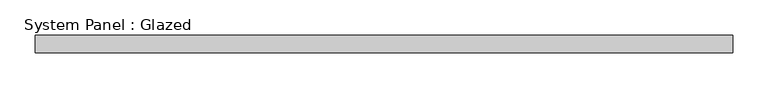
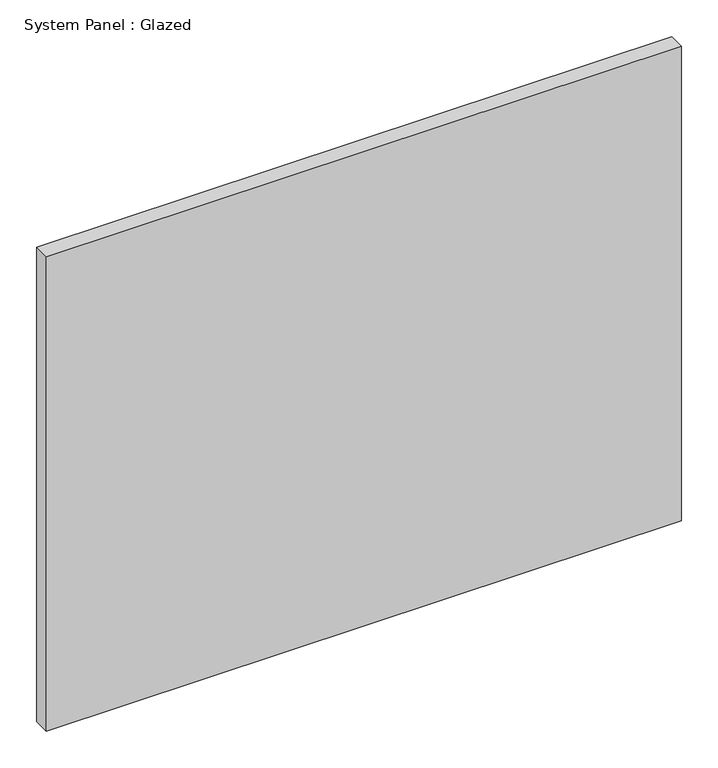
"""IFC4 building model written with IfcOpenShell, lengths in millimetres: plate geometry, System Panel : Glazed."""

from ifc_helpers import new_model, si_unit, origin, origin_with_axes, place, context, project, spatial, polyline, outline, extrude, source, transform, mapped, element, save


def system_panel_glazed_b223e52b(model_context):
    return source(origin(), model_context, "Body", "SweptSolid", [
        extrude(outline(polyline([(498.475, 19.05), (-498.475, 19.05), (-498.475, 44.45), (498.475, 44.45), (498.475, 19.05)])), origin_with_axes(), (0.0, 0.0, 1.0), 787.4),
    ])


if __name__ == "__main__":
    model = new_model("IFC4")
    model_context = context("Model", 3, world=origin())
    ifc_project = project(units=[si_unit("LENGTHUNIT", "METRE", prefix="MILLI")], contexts=[model_context])
    site = spatial("IfcSite", under=ifc_project)
    building = spatial("IfcBuilding", under=site)
    placement = place(None, origin())
    system_panel_glazed_shape = system_panel_glazed_b223e52b(model_context)
    element("IfcPlate", 1, ObjectType="System Panel : Glazed", at=placement, inside=building, context=model_context, shape_type="MappedRepresentation", body=[
        mapped(system_panel_glazed_shape, transform((0.0, 0.0, 0.0), x_axis=(1.0, 0.0, 0.0), y_axis=(0.0, 1.0, 0.0), z_axis=(0.0, 0.0, 1.0))),
    ])
    save(model, "model.ifc")

# Revit data of these elements
# Type "System Panel : Glazed"
#   Construction Type Id = "GSP4R"
#   Analytic Construction = "1/8 in Pilkington single glazing"
#   Visual Light Transmittance = 0.9
#   Solar Heat Gain Coefficient = 0.86
#   Heat Transfer Coefficient (U) = 1.18115 BTU/(h·ft²·°F)
# Element 1 (IfcPlate, "System Panel : Glazed")
#   Materials on its faces: "Glass"
# Materials
#   "Glass": class "Glass", colour RGB 0 128 192, transparency 0.75, Description = "Soda Lime Glass", Cost = 0
